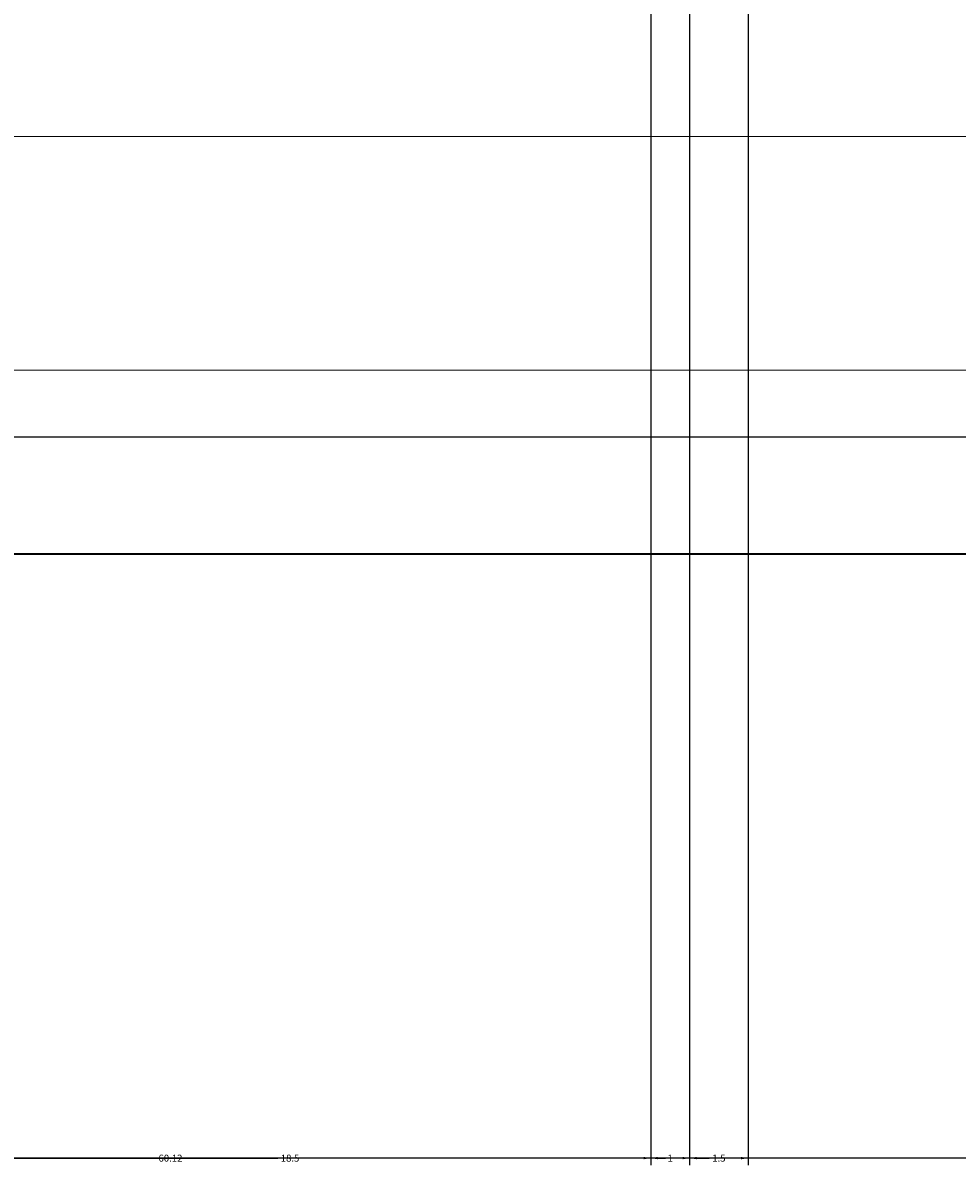
# Model space of a CAD drawing. Units: inches. Extents: x -6 to 289, y -8 to 323.
# Tile 17 of 107: x 150 to 174, y -8 to 21. Entities that reach past the tile are written whole.
import ezdxf

# ---------------------------------------------------------------- set-up
doc = ezdxf.new("R2010")
doc.units = ezdxf.units.IN
doc.header["$MEASUREMENT"] = 0
for name, color, linetype, lineweight in [('A-ANNO-DIMS', 2, 'Continuous', 18), ('A-DOOR', 3, 'Continuous', 25), ('A-ELEV', 7, 'Continuous', 35), ('A-ELEV-PATT', 8, 'Continuous', 13)]:
    doc.layers.add(name, color=color, linetype=linetype, lineweight=lineweight)
doc.styles.get("Standard").update_dxf_attribs({"font": 'arial.ttf'})
doc.dimstyles.get("Standard").update_dxf_attribs({"dimtxt": 0.18, "dimasz": 0.18, "dimexe": 0.18, "dimexo": 0.0625, "dimgap": 0.09, "dimtad": 0, "dimtih": 1, "dimtoh": 1, "dimdec": 4, "dimzin": 0, "dimdsep": 46, "dimtxsty": 'Standard', "dimcen": 0.09, "dimadec": 0, "dimazin": 0, "dimtfac": 1, "dimtdec": 4, "dimtofl": 0, "dimtmove": 0, "dimatfit": 3, "dimfxl": 1, "dimtolj": 1, "dimtzin": 0, "dimarcsym": 0})

# ---------------------------------------------------------------- blocks, each defined once
blk = doc.blocks.new('*D16')
at = {"layer": 'A-ANNO-DIMS', "color": 0, "lineweight": -2, "transparency": 16777216}
for p, q in [((9.943, 68.37), (9.943, -8.391)), ((272.973, 68.37), (272.973, -8.391)), ((10.123, -8.211), (140.993, -8.211)), ((272.793, -8.211), (141.923, -8.211))]:
    blk.add_line(p, q, dxfattribs=at)
at = {"layer": 'A-ANNO-DIMS', "color": 0, "transparency": 16777216}
for points in [[(10.123, -8.181), (10.123, -8.241), (9.943, -8.211)], [(272.793, -8.181), (272.793, -8.241), (272.973, -8.211)]]:
    blk.add_solid(points, dxfattribs=at)
at = {"layer": 'Defpoints', "color": 0, "transparency": 16777216}
for p in [(9.943, 68.432), (272.973, 68.432), (272.973, -8.211)]:
    blk.add_point(p, dxfattribs=at)
at = {"layer": 'A-ANNO-DIMS', "color": 0, "transparency": 16777216, "insert": (141.458, -8.211), "char_height": 0.18, "attachment_point": 5}
blk.add_mtext('\\A1;263.03', dxfattribs=at)
blk = doc.blocks.new('*D32')
at = {"layer": 'A-ANNO-DIMS', "color": 0, "lineweight": -2, "transparency": 16777216}
for p, q in [((147.883, 181.092), (147.883, -8.391)), ((166.383, 181.092), (166.383, -8.391)), ((148.063, -8.211), (156.817, -8.211)), ((166.203, -8.211), (157.449, -8.211))]:
    blk.add_line(p, q, dxfattribs=at)
at = {"layer": 'A-ANNO-DIMS', "color": 0, "transparency": 16777216}
for points in [[(148.063, -8.181), (148.063, -8.241), (147.883, -8.211)], [(166.203, -8.181), (166.203, -8.241), (166.383, -8.211)]]:
    blk.add_solid(points, dxfattribs=at)
at = {"layer": 'Defpoints', "color": 0, "transparency": 16777216}
for p in [(147.883, 181.154), (166.383, 181.154), (166.383, -8.211)]:
    blk.add_point(p, dxfattribs=at)
at = {"layer": 'A-ANNO-DIMS', "color": 0, "transparency": 16777216, "insert": (157.133, -8.211), "char_height": 0.18, "attachment_point": 5}
blk.add_mtext('\\A1;18.5', dxfattribs=at)
blk = doc.blocks.new('*D33')
at = {"layer": 'A-ANNO-DIMS', "color": 0, "lineweight": -2, "transparency": 16777216}
for p, q in [((166.383, 181.092), (166.383, -8.391)), ((167.383, 180.092), (167.383, -8.391)), ((166.563, -8.211), (166.76, -8.211)), ((167.203, -8.211), (167.007, -8.211))]:
    blk.add_line(p, q, dxfattribs=at)
at = {"layer": 'A-ANNO-DIMS', "color": 0, "transparency": 16777216}
for points in [[(166.563, -8.181), (166.563, -8.241), (166.383, -8.211)], [(167.203, -8.181), (167.203, -8.241), (167.383, -8.211)]]:
    blk.add_solid(points, dxfattribs=at)
at = {"layer": 'Defpoints', "color": 0, "transparency": 16777216}
for p in [(166.383, 181.154), (167.383, 180.154), (167.383, -8.211)]:
    blk.add_point(p, dxfattribs=at)
at = {"layer": 'A-ANNO-DIMS', "color": 0, "transparency": 16777216, "insert": (166.883, -8.211), "char_height": 0.18, "attachment_point": 5}
blk.add_mtext('\\A1;1', dxfattribs=at)
blk = doc.blocks.new('*D34')
at = {"layer": 'A-ANNO-DIMS', "color": 0, "lineweight": -2, "transparency": 16777216}
for p, q in [((167.383, 180.092), (167.383, -8.391)), ((168.883, 178.592), (168.883, -8.391)), ((167.563, -8.211), (167.887, -8.211)), ((168.703, -8.211), (168.38, -8.211))]:
    blk.add_line(p, q, dxfattribs=at)
at = {"layer": 'A-ANNO-DIMS', "color": 0, "transparency": 16777216}
for points in [[(167.563, -8.181), (167.563, -8.241), (167.383, -8.211)], [(168.703, -8.181), (168.703, -8.241), (168.883, -8.211)]]:
    blk.add_solid(points, dxfattribs=at)
at = {"layer": 'Defpoints', "color": 0, "transparency": 16777216}
for p in [(167.383, 180.154), (168.883, 178.654), (168.883, -8.211)]:
    blk.add_point(p, dxfattribs=at)
at = {"layer": 'A-ANNO-DIMS', "color": 0, "transparency": 16777216, "insert": (168.133, -8.211), "char_height": 0.18, "attachment_point": 5}
blk.add_mtext('\\A1;1.5', dxfattribs=at)
blk = doc.blocks.new('*D68')
at = {"layer": 'A-ANNO-DIMS', "color": 0, "lineweight": -2, "transparency": 16777216}
for p, q in [((124.008, 10.226), (124.008, -8.391)), ((184.124, 10.226), (184.124, -8.391)), ((124.188, -8.211), (153.673, -8.211)), ((183.944, -8.211), (154.459, -8.211))]:
    blk.add_line(p, q, dxfattribs=at)
at = {"layer": 'A-ANNO-DIMS', "color": 0, "transparency": 16777216}
for points in [[(124.188, -8.181), (124.188, -8.241), (124.008, -8.211)], [(183.944, -8.181), (183.944, -8.241), (184.124, -8.211)]]:
    blk.add_solid(points, dxfattribs=at)
at = {"layer": 'Defpoints', "color": 0, "transparency": 16777216}
for p in [(124.008, 10.289), (184.124, 10.289), (184.124, -8.211)]:
    blk.add_point(p, dxfattribs=at)
at = {"layer": 'A-ANNO-DIMS', "color": 0, "transparency": 16777216, "insert": (154.066, -8.211), "char_height": 0.18, "attachment_point": 5}
blk.add_mtext('\\A1;60.12', dxfattribs=at)

msp = doc.modelspace()

# ---------------------------------------------------------------- hatches: boundary and pattern name
at = {"layer": 'A-ELEV-PATT'}
h = msp.add_hatch(dxfattribs=at)
h.set_pattern_fill('_USER', color=256, scale=6, pattern_type=0)
h.set_pattern_definition([(0, (0, 0), (0, 6), [])])
h.paths.add_polyline_path([(184.1244, 48.0851), (124.008, 48.0851), (124.008, 10.2888), (184.1244, 10.2888)])
h.paths.add_polyline_path([(244.2408, 48.0851), (186.3604, 48.0851), (186.3604, 10.2888), (244.2408, 10.2888)])
h.paths.add_polyline_path([(208.2918, 114.2795), (190.7918, 114.2795), (190.7918, 71.2795), (208.2918, 71.2795)])
h.paths.add_polyline_path([(227.7918, 114.2795), (209.2918, 114.2795), (209.2918, 71.2795), (227.7918, 71.2795)])
h.paths.add_polyline_path([(211.2918, 224.3887), (190.7918, 224.3887), (190.7918, 162.3484), (211.2918, 162.3484)])
h.paths.add_polyline_path([(233.7918, 224.3887), (212.2918, 224.3887), (212.2918, 162.3484), (233.7918, 162.3484)])
h.paths.add_polyline_path([(166.3835, 224.154), (147.8835, 224.154), (147.8835, 181.154), (166.3835, 181.154)])
h.paths.add_polyline_path([(146.8835, 224.154), (129.3835, 224.154), (129.3835, 181.154), (146.8835, 181.154)])

# ---------------------------------------------------------------- linework, layer by layer
at = {"layer": 'A-DOOR'}
for points in [[(121.008, 51.0851), (247.2408, 51.0851), (247.2408, 7.2888), (121.008, 7.2888)], [(124.008, 48.0851), (244.2408, 48.0851), (244.2408, 10.2888), (124.008, 10.2888)]]:
    msp.add_lwpolyline(points, close=True, dxfattribs=at)
at = {"layer": 'A-ELEV'}
msp.add_line((19.1638, 7.2888), (271.1638, 7.2888), dxfattribs=at)

# ---------------------------------------------------------------- dimensions: what is measured, and where the dimension line sits
at = {"layer": 'A-ANNO-DIMS'}
for base, p1, p2, override, picture, middle in [((166.3835, -8.2112), (147.8835, 181.154), (166.3835, 181.154), {"dimdec": 1, "dimlfac": 1, "dimrnd": 0, "dimzin": 0, "dimdsep": 46, "dimlunit": 2}, '*D32', (157.1335, -8.2112)), ((167.3835, -8.2112), (166.3835, 181.154), (167.3835, 180.154), {"dimdec": 0, "dimlfac": 1, "dimrnd": 0, "dimzin": 0, "dimdsep": 46, "dimlunit": 2}, '*D33', (166.8835, -8.2112)), ((168.8835, -8.2112), (167.3835, 180.154), (168.8835, 178.654), {"dimdec": 1, "dimlfac": 1, "dimrnd": 0, "dimzin": 0, "dimdsep": 46, "dimlunit": 2}, '*D34', (168.1335, -8.2112)), ((272.9733, -8.2112), (9.943, 68.4322), (272.9733, 68.4322), {"dimdec": 2, "dimlfac": 1, "dimrnd": 0, "dimzin": 0, "dimdsep": 46, "dimlunit": 2}, '*D16', (141.4581, -8.2112)), ((184.1244, -8.2112), (124.008, 10.2888), (184.1244, 10.2888), {"dimdec": 2, "dimlfac": 1, "dimrnd": 0, "dimzin": 0, "dimdsep": 46, "dimlunit": 2}, '*D68', (154.0662, -8.2112))]:
    dim = msp.add_linear_dim(base=base, p1=p1, p2=p2, dimstyle='Standard', override=override, dxfattribs=at)
    dim.commit()
    dim.dimension.update_dxf_attribs({"geometry": picture, "text_midpoint": middle})

doc.saveas('drawing.dxf')
